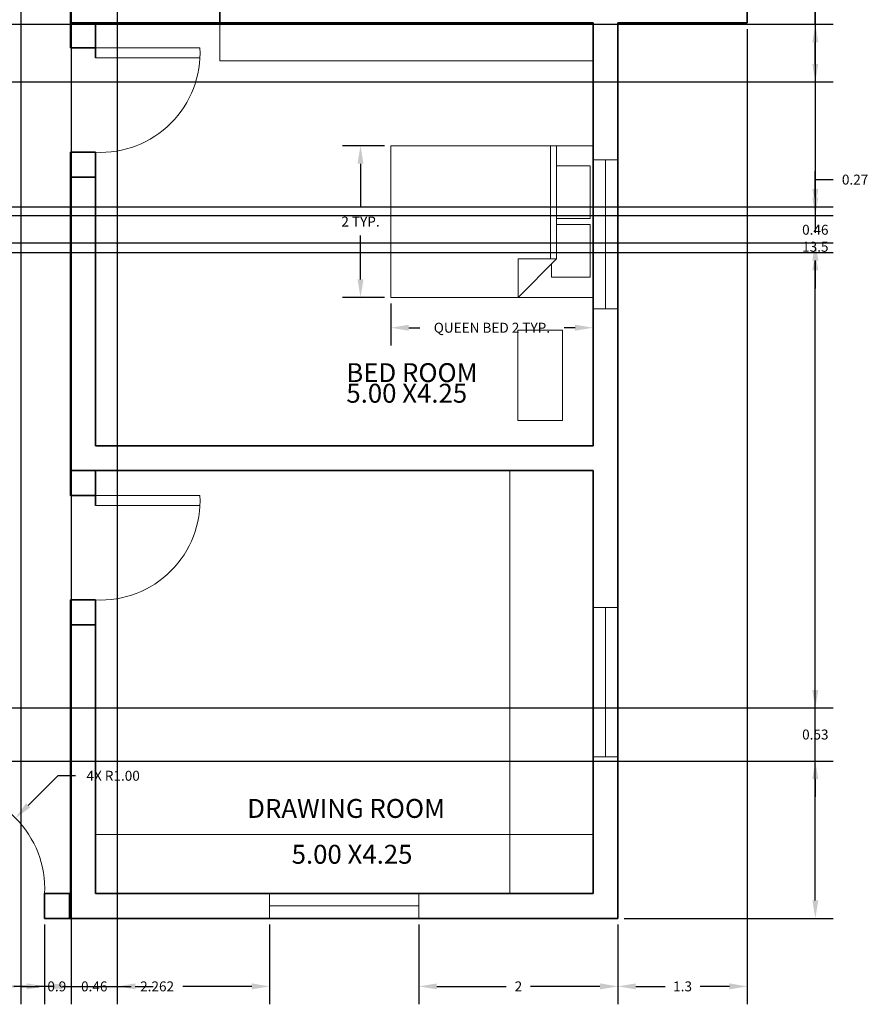
# Model space of a CAD drawing. Units: metres. Extents: x 180.3 to 196.1, y 135.7 to 166.1.
# Tile 4 of 5: x 187.5 to 196.1, y 150.9 to 160.8. Entities that reach past the tile are written whole.
import ezdxf

# ---------------------------------------------------------------- set-up
doc = ezdxf.new("R2010")
doc.units = ezdxf.units.M
doc.header["$MEASUREMENT"] = 0
for name, color, linetype, lineweight in [('A-ANNO-DIMS', 2, 'Continuous', 18), ('A-AREA-IDEN', 210, 'Continuous', 18), ('A-FLOR-CASE', 8, 'Continuous', 18), ('A-FURN', 190, 'Continuous', 18), ('A-GLAZ', 130, 'Continuous', 18), ('dim', 70, 'Continuous', 15), ('door', 240, 'Continuous', 18), ('wall', 50, 'Continuous', 35)]:
    doc.layers.add(name, color=color, linetype=linetype, lineweight=lineweight)
doc.styles.get("Standard").update_dxf_attribs({"font": 'arial.ttf', "height": 0.1})
doc.dimstyles.get("Standard").update_dxf_attribs({"dimtxt": 0.18, "dimasz": 0.18, "dimexe": 0.18, "dimexo": 0.0625, "dimgap": 0.09, "dimtad": 0, "dimtih": 1, "dimtoh": 1, "dimdec": 4, "dimzin": 0, "dimdsep": 46, "dimtxsty": 'Standard', "dimcen": 0.09, "dimadec": 0, "dimazin": 0, "dimtfac": 1, "dimtdec": 4, "dimtofl": 0, "dimtmove": 0, "dimatfit": 3, "dimfxl": 1, "dimtolj": 1, "dimtzin": 0, "dimarcsym": 0})

# ---------------------------------------------------------------- blocks, each defined once
blk = doc.blocks.new('Bed - Queen')
for p, q in [((0, -80.00003), (0, 0)), ((0, 0), (59.99999, 0)), ((59.99999, 0), (59.99999, -80.00003)), ((7.99999, -1.2), (28.79998, -1.2)), ((7.99999, -14.4), (7.99999, -1.2)), ((28.79998, -1.2), (28.79998, -14.4)), ((31.19999, -1.2), (51.99999, -1.2)), ((31.19999, -14.4), (31.19999, -1.2)), ((51.99999, -1.2), (51.99999, -16.4)), ((0, -14.4), (44.8, -14.4)), ((59.99999, -29.6), (44.8, -14.4)), ((44.8, -14.4), (44.8, -29.6)), ((44.8, -16.8), (0, -16.8)), ((51.99999, -16.4), (46.79936, -16.4)), ((44.8, -29.6), (59.99999, -29.6)), ((59.99999, -80.00003), (0, -80.00003))]:
    blk.add_line(p, q)
blk = doc.blocks.new('DOOR-1050')
for p, q in [((0.0004, -0.0001), (0.0004, 1.0499)), ((0.1004, -0.0001), (0.1004, 1.0499))]:
    blk.add_line(p, q)
blk.add_arc((0.0504, 0.0499), 1.0012, 357.13759, 92.86241)
blk = doc.blocks.new('WIN-1500')
for p, q in [((0.0003, 0.2499), (0.0003, -0.0001)), ((1.5003, 0.2499), (1.5003, -0.0001)), ((1.5003, 0.1249), (0.0003, 0.1249))]:
    blk.add_line(p, q)
blk = doc.blocks.new('*D21')
at = {"layer": 'A-ANNO-DIMS', "color": 0, "lineweight": -2, "transparency": 16777216}
for p, q in [((191.2653, 157.9265), (191.2653, 157.5042)), ((193.2973, 157.9265), (193.2973, 157.5042)), ((191.4453, 157.6842), (191.5561, 157.6842)), ((193.1173, 157.6842), (193.0066, 157.6842))]:
    blk.add_line(p, q, dxfattribs=at)
at = {"layer": 'A-ANNO-DIMS', "color": 0, "transparency": 16777216}
for points in [[(191.4453, 157.7142), (191.4453, 157.6542), (191.2653, 157.6842)], [(193.1173, 157.7142), (193.1173, 157.6542), (193.2973, 157.6842)]]:
    blk.add_solid(points, dxfattribs=at)
at = {"layer": 'Defpoints', "color": 0, "transparency": 16777216}
for p in [(191.2653, 157.989), (193.2973, 157.989), (193.2973, 157.6842)]:
    blk.add_point(p, dxfattribs=at)
at = {"layer": 'A-ANNO-DIMS', "color": 0, "transparency": 16777216, "insert": (192.2813, 157.6842), "char_height": 0.1, "attachment_point": 5}
blk.add_mtext('\\A1;QUEEN BED 2 TYP.', dxfattribs=at)
blk = doc.blocks.new('*D22')
at = {"layer": 'A-ANNO-DIMS', "color": 0, "lineweight": -2, "transparency": 16777216}
for p, q in [((191.2028, 159.513), (190.7805, 159.513)), ((190.9605, 159.333), (190.9605, 158.8913)), ((190.9605, 158.169), (190.9605, 158.6108)), ((191.2028, 157.989), (190.7805, 157.989))]:
    blk.add_line(p, q, dxfattribs=at)
at = {"layer": 'A-ANNO-DIMS', "color": 0, "transparency": 16777216}
for points in [[(190.9305, 159.333), (190.9905, 159.333), (190.9605, 159.513)], [(190.9305, 158.169), (190.9905, 158.169), (190.9605, 157.989)]]:
    blk.add_solid(points, dxfattribs=at)
at = {"layer": 'Defpoints', "color": 0, "transparency": 16777216}
for p in [(191.2653, 159.513), (190.9605, 157.989), (191.2653, 157.989)]:
    blk.add_point(p, dxfattribs=at)
at = {"layer": 'A-ANNO-DIMS', "color": 0, "transparency": 16777216, "insert": (190.9605, 158.751), "char_height": 0.1, "attachment_point": 5}
blk.add_mtext('\\A1;2 TYP.', dxfattribs=at)
blk = doc.blocks.new('*D33')
at = {"layer": 'A-ANNO-DIMS', "color": 0, "lineweight": -2, "transparency": 16777216}
for p, q in [((181.1973, 156.5604), (181.1973, 166.1117)), ((194.8473, 160.8104), (194.8473, 166.1117)), ((181.3773, 165.9317), (187.7679, 165.9317)), ((194.6673, 165.9317), (188.2767, 165.9317))]:
    blk.add_line(p, q, dxfattribs=at)
at = {"layer": 'A-ANNO-DIMS', "color": 0, "transparency": 16777216}
for points in [[(181.3773, 165.9617), (181.3773, 165.9017), (181.1973, 165.9317)], [(194.6673, 165.9617), (194.6673, 165.9017), (194.8473, 165.9317)]]:
    blk.add_solid(points, dxfattribs=at)
at = {"layer": 'Defpoints', "color": 0, "transparency": 16777216}
for p in [(194.8473, 165.9317), (194.8473, 160.7479), (181.1973, 156.4979)]:
    blk.add_point(p, dxfattribs=at)
at = {"layer": 'A-ANNO-DIMS', "color": 0, "transparency": 16777216, "insert": (188.0223, 165.9317), "char_height": 0.1, "attachment_point": 5}
blk.add_mtext('\\A1;13.65', dxfattribs=at)
blk = doc.blocks.new('*D34')
at = {"layer": 'A-ANNO-DIMS', "color": 0, "lineweight": -2, "transparency": 16777216}
for p, q in [((194.9098, 165.2479), (195.7111, 165.2479)), ((195.5311, 165.0679), (195.5311, 158.639)), ((195.5311, 151.9279), (195.5311, 158.3568)), ((193.6098, 151.7479), (195.7111, 151.7479))]:
    blk.add_line(p, q, dxfattribs=at)
at = {"layer": 'A-ANNO-DIMS', "color": 0, "transparency": 16777216}
for points in [[(195.5011, 165.0679), (195.5611, 165.0679), (195.5311, 165.2479)], [(195.5011, 151.9279), (195.5611, 151.9279), (195.5311, 151.7479)]]:
    blk.add_solid(points, dxfattribs=at)
at = {"layer": 'Defpoints', "color": 0, "transparency": 16777216}
for p in [(194.8473, 165.2479), (195.5311, 165.2479), (193.5473, 151.7479)]:
    blk.add_point(p, dxfattribs=at)
at = {"layer": 'A-ANNO-DIMS', "color": 0, "transparency": 16777216, "insert": (195.5311, 158.4979), "char_height": 0.1, "attachment_point": 5}
blk.add_mtext('\\A1;13.5', dxfattribs=at)
blk = doc.blocks.new('*D37')
at = {"layer": 'A-ANNO-DIMS', "color": 0, "lineweight": -2, "transparency": 16777216}
for p, q in [((194.8473, 160.6854), (194.8473, 150.8842)), ((193.5473, 151.6854), (193.5473, 150.8842)), ((193.7273, 151.0642), (194.021, 151.0642)), ((194.6673, 151.0642), (194.3737, 151.0642))]:
    blk.add_line(p, q, dxfattribs=at)
at = {"layer": 'A-ANNO-DIMS', "color": 0, "transparency": 16777216}
for points in [[(193.7273, 151.0942), (193.7273, 151.0342), (193.5473, 151.0642)], [(194.6673, 151.0942), (194.6673, 151.0342), (194.8473, 151.0642)]]:
    blk.add_solid(points, dxfattribs=at)
at = {"layer": 'Defpoints', "color": 0, "transparency": 16777216}
for p in [(194.8473, 160.7479), (193.5473, 151.7479), (194.8473, 151.0642)]:
    blk.add_point(p, dxfattribs=at)
at = {"layer": 'A-ANNO-DIMS', "color": 0, "transparency": 16777216, "insert": (194.1973, 151.0642), "char_height": 0.1, "attachment_point": 5}
blk.add_mtext('\\A1;1.3', dxfattribs=at)
blk = doc.blocks.new('*D42')
at = {"layer": 'A-ANNO-DIMS', "color": 0, "lineweight": -2, "transparency": 16777216}
for p, q in [((186.7354, 151.6854), (186.7354, 150.8842)), ((187.7854, 151.6854), (187.7854, 150.8842)), ((186.9154, 151.0642), (187.0449, 151.0642)), ((187.6054, 151.0642), (187.476, 151.0642))]:
    blk.add_line(p, q, dxfattribs=at)
at = {"layer": 'A-ANNO-DIMS', "color": 0, "transparency": 16777216}
for points in [[(186.9154, 151.0942), (186.9154, 151.0342), (186.7354, 151.0642)], [(187.6054, 151.0942), (187.6054, 151.0342), (187.7854, 151.0642)]]:
    blk.add_solid(points, dxfattribs=at)
at = {"layer": 'Defpoints', "color": 0, "transparency": 16777216}
for p in [(186.7354, 151.7479), (187.7854, 151.7479), (187.7854, 151.0642)]:
    blk.add_point(p, dxfattribs=at)
at = {"layer": 'A-ANNO-DIMS', "color": 0, "transparency": 16777216, "insert": (187.2604, 151.0642), "char_height": 0.1, "attachment_point": 5}
blk.add_mtext('\\A1;1.05', dxfattribs=at)
blk = doc.blocks.new('*D43')
at = {"layer": 'A-ANNO-DIMS', "color": 0, "lineweight": -2, "transparency": 16777216}
for p, q in [((187.7854, 151.6854), (187.7854, 150.8842)), ((190.0473, 151.6854), (190.0473, 150.8842)), ((187.9654, 151.0642), (188.6573, 151.0642)), ((189.8673, 151.0642), (189.1754, 151.0642))]:
    blk.add_line(p, q, dxfattribs=at)
at = {"layer": 'A-ANNO-DIMS', "color": 0, "transparency": 16777216}
for points in [[(187.9654, 151.0942), (187.9654, 151.0342), (187.7854, 151.0642)], [(189.8673, 151.0942), (189.8673, 151.0342), (190.0473, 151.0642)]]:
    blk.add_solid(points, dxfattribs=at)
at = {"layer": 'Defpoints', "color": 0, "transparency": 16777216}
for p in [(187.7854, 151.7479), (190.0473, 151.7479), (190.0473, 151.0642)]:
    blk.add_point(p, dxfattribs=at)
at = {"layer": 'A-ANNO-DIMS', "color": 0, "transparency": 16777216, "insert": (188.9164, 151.0642), "char_height": 0.1, "attachment_point": 5}
blk.add_mtext('\\A1;2.262', dxfattribs=at)
blk = doc.blocks.new('*D44')
at = {"layer": 'A-ANNO-DIMS', "color": 0, "lineweight": -2, "transparency": 16777216}
for p, q in [((191.5473, 151.6854), (191.5473, 150.8842)), ((193.5473, 151.6854), (193.5473, 150.8842)), ((191.7273, 151.0642), (192.4242, 151.0642)), ((193.3673, 151.0642), (192.6705, 151.0642))]:
    blk.add_line(p, q, dxfattribs=at)
at = {"layer": 'A-ANNO-DIMS', "color": 0, "transparency": 16777216}
for points in [[(191.7273, 151.0942), (191.7273, 151.0342), (191.5473, 151.0642)], [(193.3673, 151.0942), (193.3673, 151.0342), (193.5473, 151.0642)]]:
    blk.add_solid(points, dxfattribs=at)
at = {"layer": 'Defpoints', "color": 0, "transparency": 16777216}
for p in [(191.5473, 151.7479), (193.5473, 151.7479), (193.5473, 151.0642)]:
    blk.add_point(p, dxfattribs=at)
at = {"layer": 'A-ANNO-DIMS', "color": 0, "transparency": 16777216, "insert": (192.5473, 151.0642), "char_height": 0.1, "attachment_point": 5}
blk.add_mtext('\\A1;2', dxfattribs=at)
blk = doc.blocks.new('*D53')
at = {"layer": 'A-ANNO-DIMS', "color": 0, "lineweight": -2, "transparency": 16777216}
for p, q in [((195.531085, 159.077902), (195.531085, 159.257902)), ((184.57756, 158.897902), (195.711085, 158.897902)), ((184.57756, 158.43968), (195.711085, 158.43968)), ((195.531085, 158.25968), (195.531085, 158.07968))]:
    blk.add_line(p, q, dxfattribs=at)
at = {"layer": 'A-ANNO-DIMS', "color": 0, "transparency": 16777216}
for points in [[(195.501085, 159.077902), (195.561085, 159.077902), (195.531085, 158.897902)], [(195.501085, 158.25968), (195.561085, 158.25968), (195.531085, 158.43968)]]:
    blk.add_solid(points, dxfattribs=at)
at = {"layer": 'Defpoints', "color": 0, "transparency": 16777216}
for p in [(184.51506, 158.897902), (195.531085, 158.897902), (184.51506, 158.43968)]:
    blk.add_point(p, dxfattribs=at)
at = {"layer": 'A-ANNO-DIMS', "color": 0, "transparency": 16777216, "insert": (195.531085, 158.668791), "char_height": 0.1, "attachment_point": 5}
blk.add_mtext('\\A1;0.46', dxfattribs=at)
blk = doc.blocks.new('*D54')
at = {"layer": 'A-ANNO-DIMS', "color": 0, "lineweight": -2, "transparency": 16777216}
for p, q in [((186.6473, 162.1854), (186.6473, 150.8842)), ((187.5473, 162.1854), (187.5473, 150.8842)), ((186.8273, 151.0642), (187.3673, 151.0642)), ((187.5473, 151.0642), (187.7273, 151.0642))]:
    blk.add_line(p, q, dxfattribs=at)
at = {"layer": 'A-ANNO-DIMS', "color": 0, "transparency": 16777216}
for points in [[(186.8273, 151.0942), (186.8273, 151.0342), (186.6473, 151.0642)], [(187.3673, 151.0942), (187.3673, 151.0342), (187.5473, 151.0642)]]:
    blk.add_solid(points, dxfattribs=at)
at = {"layer": 'Defpoints', "color": 0, "transparency": 16777216}
for p in [(186.6473, 162.2479), (187.5473, 162.2479), (187.5473, 151.0642)]:
    blk.add_point(p, dxfattribs=at)
at = {"layer": 'A-ANNO-DIMS', "color": 0, "transparency": 16777216, "insert": (187.9085, 151.0642), "char_height": 0.1, "attachment_point": 5}
blk.add_mtext('\\A1;0.9', dxfattribs=at)
blk = doc.blocks.new('*D57')
at = {"layer": 'A-ANNO-DIMS', "color": 0, "lineweight": -2, "transparency": 16777216}
for p, q in [((188.0529, 163.2328), (188.0529, 150.8842)), ((188.5166, 163.2178), (188.5166, 150.8842)), ((187.8729, 151.0642), (187.6929, 151.0642)), ((188.6966, 151.0642), (188.8766, 151.0642))]:
    blk.add_line(p, q, dxfattribs=at)
at = {"layer": 'A-ANNO-DIMS', "color": 0, "transparency": 16777216}
for points in [[(187.8729, 151.0942), (187.8729, 151.0342), (188.0529, 151.0642)], [(188.6966, 151.0942), (188.6966, 151.0342), (188.5166, 151.0642)]]:
    blk.add_solid(points, dxfattribs=at)
at = {"layer": 'Defpoints', "color": 0, "transparency": 16777216}
for p in [(188.0529, 163.2953), (188.5166, 163.2803), (188.5166, 151.0642)]:
    blk.add_point(p, dxfattribs=at)
at = {"layer": 'A-ANNO-DIMS', "color": 0, "transparency": 16777216, "insert": (188.2848, 151.0642), "char_height": 0.1, "attachment_point": 5}
blk.add_mtext('\\A1;0.46', dxfattribs=at)
blk = doc.blocks.new('*D60')
at = {"layer": 'A-ANNO-DIMS', "color": 0, "lineweight": -2, "transparency": 16777216}
for p, q in [((195.5311, 160.7337), (195.5311, 160.9137)), ((195.5311, 160.9137), (195.7111, 160.9137)), ((184.3834, 160.7337), (195.7111, 160.7337)), ((195.5311, 160.3348), (195.5311, 160.5537)), ((184.3647, 160.1548), (195.7111, 160.1548))]:
    blk.add_line(p, q, dxfattribs=at)
at = {"layer": 'A-ANNO-DIMS', "color": 0, "transparency": 16777216}
for points in [[(195.5011, 160.5537), (195.5611, 160.5537), (195.5311, 160.7337)], [(195.5011, 160.3348), (195.5611, 160.3348), (195.5311, 160.1548)]]:
    blk.add_solid(points, dxfattribs=at)
at = {"layer": 'Defpoints', "color": 0, "transparency": 16777216}
for p in [(184.3209, 160.7337), (195.5311, 160.7337), (184.3022, 160.1548)]:
    blk.add_point(p, dxfattribs=at)
at = {"layer": 'A-ANNO-DIMS', "color": 0, "transparency": 16777216, "insert": (195.9311, 160.9137), "char_height": 0.1, "attachment_point": 5}
blk.add_mtext('\\A1;0.58', dxfattribs=at)
blk = doc.blocks.new('*D62')
at = {"layer": 'A-ANNO-DIMS', "color": 0, "lineweight": -2, "transparency": 16777216}
for p, q in [((195.5311, 158.9929), (195.5311, 159.1729)), ((195.5311, 159.1729), (195.7111, 159.1729)), ((184.0771, 158.8129), (195.7111, 158.8129)), ((184.0771, 158.539), (195.7111, 158.539)), ((195.5311, 158.359), (195.5311, 158.179))]:
    blk.add_line(p, q, dxfattribs=at)
at = {"layer": 'A-ANNO-DIMS', "color": 0, "transparency": 16777216}
for points in [[(195.5011, 158.9929), (195.5611, 158.9929), (195.5311, 158.8129)], [(195.5011, 158.359), (195.5611, 158.359), (195.5311, 158.539)]]:
    blk.add_solid(points, dxfattribs=at)
at = {"layer": 'Defpoints', "color": 0, "transparency": 16777216}
for p in [(184.0146, 158.8129), (195.5311, 158.8129), (184.0146, 158.539)]:
    blk.add_point(p, dxfattribs=at)
at = {"layer": 'A-ANNO-DIMS', "color": 0, "transparency": 16777216, "insert": (195.931, 159.1729), "char_height": 0.1, "attachment_point": 5}
blk.add_mtext('\\A1;0.27', dxfattribs=at)
blk = doc.blocks.new('*D64')
at = {"layer": 'A-ANNO-DIMS', "color": 0, "lineweight": -2, "transparency": 16777216}
for p, q in [((195.531085, 154.042344), (195.531085, 154.222344)), ((185.951216, 153.862344), (195.711085, 153.862344)), ((185.953765, 153.32895), (195.711085, 153.32895)), ((195.531085, 153.14895), (195.531085, 152.96895))]:
    blk.add_line(p, q, dxfattribs=at)
at = {"layer": 'A-ANNO-DIMS', "color": 0, "transparency": 16777216}
for points in [[(195.501085, 154.042344), (195.561085, 154.042344), (195.531085, 153.862344)], [(195.501085, 153.14895), (195.561085, 153.14895), (195.531085, 153.32895)]]:
    blk.add_solid(points, dxfattribs=at)
at = {"layer": 'Defpoints', "color": 0, "transparency": 16777216}
for p in [(185.888716, 153.862344), (195.531085, 153.862344), (185.891265, 153.32895)]:
    blk.add_point(p, dxfattribs=at)
at = {"layer": 'A-ANNO-DIMS', "color": 0, "transparency": 16777216, "insert": (195.531085, 153.595647), "char_height": 0.1, "attachment_point": 5}
blk.add_mtext('\\A1;0.53', dxfattribs=at)
blk = doc.blocks.new('*D66')
at = {"layer": 'A-ANNO-DIMS', "color": 0, "lineweight": -2, "transparency": 16777216}
for p, q in [((187.9178, 153.1811), (187.6204, 152.8835)), ((188.0978, 153.1811), (187.9178, 153.1811)), ((186.7854, 151.9579), (186.7854, 152.1379)), ((186.6954, 152.0479), (186.8754, 152.0479))]:
    blk.add_line(p, q, dxfattribs=at)
at = {"layer": 'A-ANNO-DIMS', "color": 0, "transparency": 16777216}
blk.add_solid([(187.5992, 152.9047), (187.6416, 152.8623), (187.4932, 152.7562)], dxfattribs=at)
at = {"layer": 'Defpoints', "color": 0, "transparency": 16777216}
for p in [(187.4932, 152.7562), (186.7854, 152.0479)]:
    blk.add_point(p, dxfattribs=at)
at = {"layer": 'A-ANNO-DIMS', "color": 0, "transparency": 16777216, "insert": (188.4748, 153.1811), "char_height": 0.1, "attachment_point": 5}
blk.add_mtext('\\A1;4X R1.00', dxfattribs=at)

msp = doc.modelspace()

# ---------------------------------------------------------------- linework, layer by layer
at = {"layer": 'A-FLOR-CASE'}
for points in [[(189.5473, 160.7479), (193.2973, 160.7479), (193.2973, 160.368), (189.5473, 160.368)], [(193.2973, 156.2479), (192.4607, 156.2479), (192.4607, 151.9979), (193.2973, 151.9979)], [(188.2973, 151.9979), (193.2973, 151.9979), (193.2973, 152.5904), (188.2973, 152.5904)]]:
    msp.add_lwpolyline(points, close=True, dxfattribs=at)
at = {"layer": 'A-FURN'}
msp.add_lwpolyline([(192.5406, 157.6599), (192.9905, 157.6599), (192.9905, 156.7512), (192.5406, 156.7512)], close=True, dxfattribs=at)
at = {"layer": 'wall'}
for p, q in [((194.8473, 160.7479), (194.8473, 165.2479)), ((189.5473, 160.7479), (189.5473, 161.2479)), ((188.0473, 160.9979), (188.0473, 160.4979)), ((189.5473, 160.7479), (188.2973, 160.7479)), ((188.2973, 160.7479), (188.2973, 160.3979)), ((189.5473, 160.7479), (193.2973, 160.7479)), ((193.2973, 160.7479), (193.2973, 156.4979)), ((193.5473, 160.7479), (193.5473, 156.2479)), ((193.5473, 160.7479), (194.8473, 160.7479)), ((188.0473, 159.4479), (188.0473, 156.2479)), ((188.2973, 159.4479), (188.2973, 156.4979)), ((188.0473, 156.4979), (188.0473, 155.9979)), ((193.2973, 156.4979), (188.2973, 156.4979)), ((193.2973, 156.2479), (188.0473, 156.2479)), ((188.2973, 156.2479), (188.2973, 155.8979)), ((193.2973, 156.2479), (193.2973, 151.9979)), ((193.5473, 156.2479), (193.5473, 151.7479)), ((188.0473, 154.9479), (188.0473, 151.7479)), ((188.2973, 154.9479), (188.2973, 151.9979)), ((188.0473, 151.9979), (187.7854, 151.9979)), ((193.2973, 151.9979), (188.2973, 151.9979)), ((193.5473, 151.7479), (187.7854, 151.7479))]:
    msp.add_line(p, q, dxfattribs=at)
for points in [[(188.2973, 160.7479), (188.2973, 160.4979), (188.0473, 160.4979), (188.0473, 160.7479)], [(188.2973, 159.4479), (188.2973, 159.1979), (188.0473, 159.1979), (188.0473, 159.4479)], [(188.2973, 156.2479), (188.2973, 155.9979), (188.0473, 155.9979), (188.0473, 156.2479)], [(188.2973, 154.9479), (188.2973, 154.6979), (188.0473, 154.6979), (188.0473, 154.9479)], [(187.7854, 151.9979), (188.0354, 151.9979), (188.0354, 151.7479), (187.7854, 151.7479)]]:
    msp.add_lwpolyline(points, close=True, dxfattribs=at)

# ---------------------------------------------------------------- block references
at = {"layer": 'A-FURN', "xscale": 0.0254, "yscale": 0.0254, "zscale": 0.0254, "rotation": 270.0000000000009}
msp.add_blockref('Bed - Queen', (193.2973, 159.513), dxfattribs=at)
at = {"layer": 'A-GLAZ'}
for p, rotation in [((193.5472, 157.8726), 89.9999999999965), ((193.5472, 153.3726), 89.99999999999471)]:
    msp.add_blockref('WIN-1500', p, dxfattribs=dict(at, rotation=rotation))
msp.add_blockref('WIN-1500', (190.047, 151.748), dxfattribs=at)
at = {"layer": 'door'}
for p, rotation in [((188.2974, 160.4983), 269.9999999999984), ((188.2974, 155.9983), 269.9999999999977)]:
    msp.add_blockref('DOOR-1050', p, dxfattribs=dict(at, rotation=rotation))
msp.add_blockref('DOOR-1050', (186.735, 151.998), dxfattribs=at)

# ---------------------------------------------------------------- texts
at = {"layer": 'A-AREA-IDEN', "char_height": 0.19, "attachment_point": 1}
for s, width, insert in [('BED ROOM', 2.305817, (190.8183, 157.3276)), ('\\pxqc;DRAWING ROOM ', 3.283654, (189.1742, 152.9477))]:
    msp.add_mtext_dynamic_manual_height_columns(s, width=width, gutter_width=1, heights=[0], dxfattribs=dict(at, insert=insert))
at = {"layer": 'dim', "char_height": 0.19, "attachment_point": 1}
for insert in [(190.8183, 157.1206), (190.2687, 152.487)]:
    msp.add_mtext_dynamic_manual_height_columns('5.00 X4.25', width=1.692297, gutter_width=1, heights=[0], dxfattribs=dict(at, insert=insert))

# ---------------------------------------------------------------- dimensions: what is measured, and where the dimension line sits
at = {"layer": 'A-ANNO-DIMS'}
for base, p1, p2, override, picture, middle in [((194.8473, 165.9317), (181.1973, 156.4979), (194.8473, 160.7479), {"dimdec": 2, "dimlfac": 1, "dimrnd": 0, "dimzin": 0, "dimdsep": 46, "dimlunit": 2}, '*D33', (188.0223, 165.9317)), ((188.5166, 151.0642), (188.0529, 163.2953), (188.5166, 163.2803), {"dimdec": 2, "dimlfac": 1, "dimrnd": 0, "dimzin": 0, "dimdsep": 46, "dimlunit": 2}, '*D57', (188.2848, 151.0642)), ((187.5473, 151.0642), (186.6473, 162.2479), (187.5473, 162.2479), {"dimdec": 1, "dimlfac": 1, "dimrnd": 0, "dimzin": 0, "dimdsep": 46, "dimlunit": 2}, '*D54', (187.9085, 151.0642)), ((194.8473, 151.0642), (193.5473, 151.7479), (194.8473, 160.7479), {"dimdec": 1, "dimlfac": 1, "dimrnd": 0, "dimzin": 0, "dimdsep": 46, "dimlunit": 2}, '*D37', (194.1973, 151.0642)), ((187.7854, 151.0642), (186.7354, 151.7479), (187.7854, 151.7479), {"dimdec": 2, "dimlfac": 1, "dimrnd": 0, "dimzin": 0, "dimdsep": 46, "dimlunit": 2}, '*D42', (187.2604, 151.0642)), ((190.0473, 151.0642), (187.7854, 151.7479), (190.0473, 151.7479), {"dimdec": 3, "dimlfac": 1, "dimrnd": 0, "dimzin": 0, "dimdsep": 46, "dimlunit": 2}, '*D43', (188.9164, 151.0642)), ((193.5473, 151.0642), (191.5473, 151.7479), (193.5473, 151.7479), {"dimdec": 0, "dimlfac": 1, "dimrnd": 0, "dimzin": 0, "dimdsep": 46, "dimlunit": 2}, '*D44', (192.5473, 151.0642))]:
    dim = msp.add_linear_dim(base=base, p1=p1, p2=p2, dimstyle='Standard', override=override, dxfattribs=at)
    dim.commit()
    dim.dimension.update_dxf_attribs({"geometry": picture, "text_midpoint": middle})
for base, p1, p2, override, picture, middle in [((195.5311, 165.2479), (193.5473, 151.7479), (194.8473, 165.2479), {"dimdec": 1, "dimlfac": 1, "dimrnd": 0, "dimzin": 0, "dimdsep": 46, "dimlunit": 2}, '*D34', (195.5311, 158.4979)), ((195.5311, 160.7337), (184.3022, 160.1548), (184.3209, 160.7337), {"dimdec": 2, "dimlfac": 1, "dimrnd": 0, "dimzin": 0, "dimdsep": 46, "dimlunit": 2}, '*D60', (195.9311, 160.9137)), ((195.5311, 158.8129), (184.0146, 158.539), (184.0146, 158.8129), {"dimdec": 2, "dimlfac": 1, "dimrnd": 0, "dimzin": 0, "dimdsep": 46, "dimlunit": 2}, '*D62', (195.931, 159.1729)), ((195.5311, 158.8979), (184.5151, 158.4397), (184.5151, 158.8979), {"dimdec": 2, "dimlfac": 1, "dimrnd": 0, "dimzin": 0, "dimdsep": 46, "dimlunit": 2}, '*D53', (195.5311, 158.6688)), ((195.5311, 153.8623), (185.8913, 153.3289), (185.8887, 153.8623), {"dimdec": 2, "dimlfac": 1, "dimrnd": 0, "dimzin": 0, "dimdsep": 46, "dimlunit": 2}, '*D64', (195.5311, 153.5956))]:
    dim = msp.add_linear_dim(base=base, p1=p1, p2=p2, angle=90, dimstyle='Standard', override=override, dxfattribs=at)
    dim.commit()
    dim.dimension.update_dxf_attribs({"geometry": picture, "text_midpoint": middle})
for base, p1, p2, angle, text, picture, middle in [((190.9605, 157.989), (191.2653, 159.513), (191.2653, 157.989), 270, '<> TYP.', '*D22', (190.9605, 158.751)), ((193.2973, 157.6842), (191.2653, 157.989), (193.2973, 157.989), 0, 'QUEEN BED <> TYP.', '*D21', (192.2813, 157.6842))]:
    dim = msp.add_linear_dim(base=base, p1=p1, p2=p2, angle=angle, text=text, dimstyle='Standard', override={"dimdec": 0, "dimlfac": 1, "dimrnd": 0, "dimzin": 0, "dimdsep": 46, "dimlunit": 2}, dxfattribs=at)
    dim.commit()
    dim.dimension.update_dxf_attribs({"geometry": picture, "text_midpoint": middle})
dim = msp.add_radius_dim(center=(186.7854, 152.0479), mpoint=(187.4932, 152.7562), text='4X <>', dimstyle='Standard', override={"dimdec": 2, "dimlfac": 1, "dimrnd": 0, "dimzin": 0, "dimdsep": 46, "dimlunit": 2}, dxfattribs=at)
dim.commit()
dim.dimension.update_dxf_attribs({"geometry": '*D66', "text_midpoint": (188.4748, 153.1811), "dimtype": 164})

doc.saveas('drawing.dxf')
